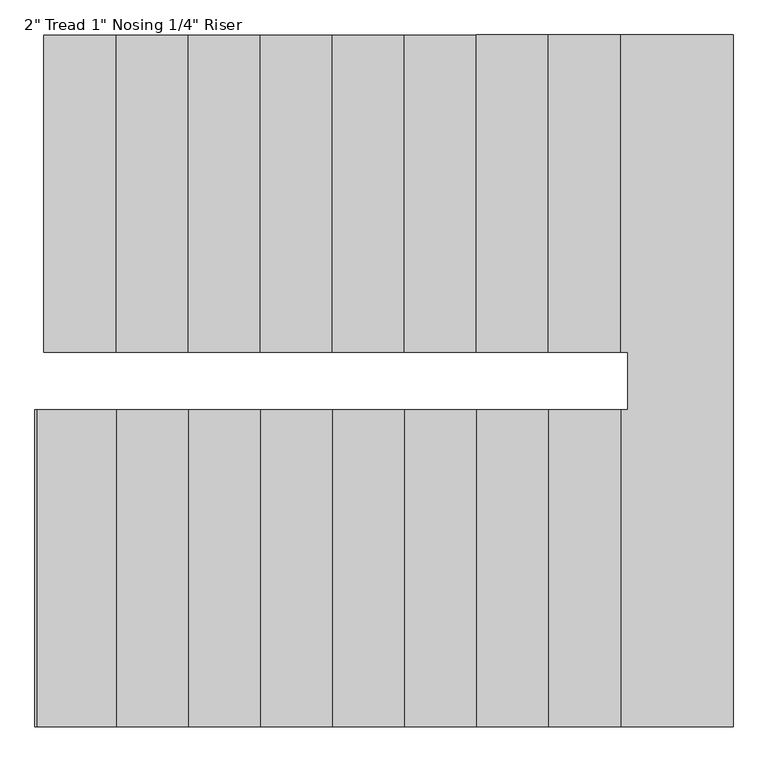
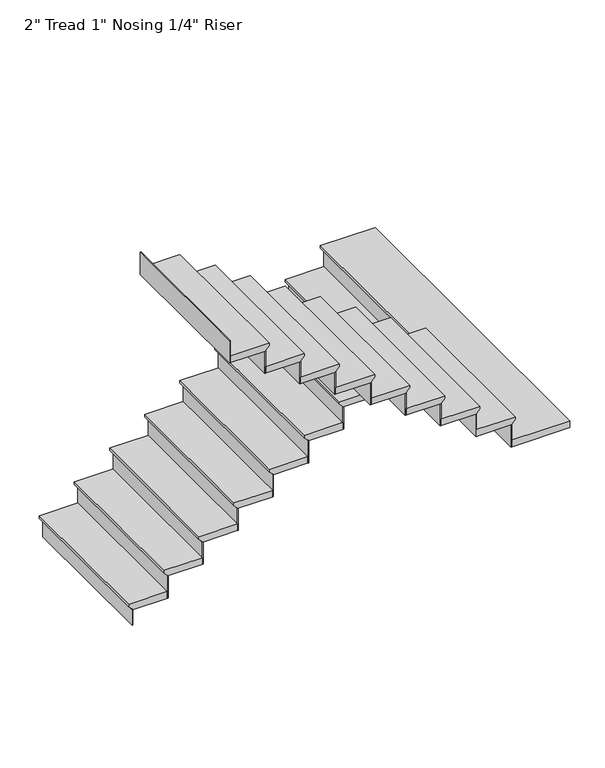
"""IFC4 building model written with IfcOpenShell, lengths in millimetres: stair flight geometry."""

from ifc_helpers import new_model, si_unit, origin, place, context, project, spatial, faceted_brep, source, transform, mapped, element, save


def stair_flight_b7e44e04(model_context):
    return source(origin(), model_context, "Body", "Brep", [
        faceted_brep([(-41148.2472477, 4654.7086027, 150.2833333), (-41148.2472477, 4654.7086027, 169.3333333), (-41148.2472477, 5772.3086027, 169.3333333), (-41148.2472477, 5772.3086027, 150.2833333), (-41122.8472477, 4654.7086027, 124.8833333), (-41122.8472477, 5772.3086027, 124.8833333), (-40868.8472477, 4654.7086027, 169.3333333), (-40868.8472477, 5772.3086027, 169.3333333), (-41122.8472477, 5772.3086027, 118.5333333), (-40868.8472477, 5772.3086027, 118.5333333), (-40868.8472477, 4654.7086027, 118.5333333), (-41122.8472477, 4654.7086027, 118.5333333)], [[[0, 1, 2, 3]], [[4, 0, 3, 5]], [[2, 1, 6, 7]], [[8, 9, 10, 11]], [[2, 7, 9, 8, 5, 3]], [[8, 11, 4, 5]], [[6, 1, 0, 4, 11, 10]], [[7, 6, 10, 9]]]),
        faceted_brep([(-41122.8472477, 4654.7086027, 118.5333333), (-41122.8472477, 4654.7086027, 0.0), (-41116.4972477, 4654.7086027, 0.0), (-41116.4972477, 4654.7086027, 118.5333333), (-41122.8472477, 5772.3086027, 118.5333333), (-41116.4972477, 5772.3086027, 118.5333333), (-41116.4972477, 5772.3086027, 0.0), (-41122.8472477, 5772.3086027, 0.0)], [[[0, 1, 2, 3]], [[4, 5, 6, 7]], [[1, 0, 4, 7]], [[2, 1, 7, 6]], [[3, 2, 6, 5]], [[0, 3, 5, 4]]]),
        faceted_brep([(-40868.8472477, 4654.7086027, 287.8666667), (-40868.8472477, 4654.7086027, 118.5333333), (-40862.4972477, 4654.7086027, 118.5333333), (-40862.4972477, 4654.7086027, 287.8666667), (-40868.8472477, 5772.3086027, 287.8666667), (-40862.4972477, 5772.3086027, 287.8666667), (-40862.4972477, 5772.3086027, 118.5333333), (-40868.8472477, 5772.3086027, 118.5333333)], [[[0, 1, 2, 3]], [[4, 5, 6, 7]], [[1, 0, 4, 7]], [[2, 1, 7, 6]], [[3, 2, 6, 5]], [[0, 3, 5, 4]]]),
        faceted_brep([(-40894.2472477, 5772.3086027, 338.6666667), (-40894.2472477, 4654.7086027, 338.6666667), (-40614.8472477, 4654.7086027, 338.6666667), (-40614.8472477, 5772.3086027, 338.6666667), (-40868.8472477, 5772.3086027, 287.8666667), (-40614.8472477, 5772.3086027, 287.8666667), (-40614.8472477, 4654.7086027, 287.8666667), (-40868.8472477, 4654.7086027, 287.8666667), (-40868.8472477, 5772.3086027, 294.2166667), (-40894.2472477, 5772.3086027, 319.6166667), (-40868.8472477, 4654.7086027, 294.2166667), (-40894.2472477, 4654.7086027, 319.6166667)], [[[0, 1, 2, 3]], [[4, 5, 6, 7]], [[0, 3, 5, 4, 8, 9]], [[4, 7, 10, 8]], [[2, 1, 11, 10, 7, 6]], [[3, 2, 6, 5]], [[11, 1, 0, 9]], [[10, 11, 9, 8]]]),
        faceted_brep([(-40614.8472477, 4654.7086027, 457.2), (-40614.8472477, 4654.7086027, 287.8666667), (-40608.4972477, 4654.7086027, 287.8666667), (-40608.4972477, 4654.7086027, 457.2), (-40614.8472477, 5772.3086027, 457.2), (-40608.4972477, 5772.3086027, 457.2), (-40608.4972477, 5772.3086027, 287.8666667), (-40614.8472477, 5772.3086027, 287.8666667)], [[[0, 1, 2, 3]], [[4, 5, 6, 7]], [[1, 0, 4, 7]], [[2, 1, 7, 6]], [[3, 2, 6, 5]], [[0, 3, 5, 4]]]),
        faceted_brep([(-40640.2472477, 5772.3086027, 508.0), (-40640.2472477, 4654.7086027, 508.0), (-40360.8472477, 4654.7086027, 508.0), (-40360.8472477, 5772.3086027, 508.0), (-40614.8472477, 5772.3086027, 457.2), (-40360.8472477, 5772.3086027, 457.2), (-40360.8472477, 4654.7086027, 457.2), (-40614.8472477, 4654.7086027, 457.2), (-40614.8472477, 5772.3086027, 463.55), (-40640.2472477, 5772.3086027, 488.95), (-40614.8472477, 4654.7086027, 463.55), (-40640.2472477, 4654.7086027, 488.95)], [[[0, 1, 2, 3]], [[4, 5, 6, 7]], [[0, 3, 5, 4, 8, 9]], [[4, 7, 10, 8]], [[2, 1, 11, 10, 7, 6]], [[3, 2, 6, 5]], [[11, 1, 0, 9]], [[10, 11, 9, 8]]]),
        faceted_brep([(-40360.8472477, 4654.7086027, 626.5333333), (-40360.8472477, 4654.7086027, 457.2), (-40354.4972477, 4654.7086027, 457.2), (-40354.4972477, 4654.7086027, 626.5333333), (-40360.8472477, 5772.3086027, 626.5333333), (-40354.4972477, 5772.3086027, 626.5333333), (-40354.4972477, 5772.3086027, 457.2), (-40360.8472477, 5772.3086027, 457.2)], [[[0, 1, 2, 3]], [[4, 5, 6, 7]], [[1, 0, 4, 7]], [[2, 1, 7, 6]], [[3, 2, 6, 5]], [[0, 3, 5, 4]]]),
        faceted_brep([(-40386.2472477, 5772.3086027, 677.3333333), (-40386.2472477, 4654.7086027, 677.3333333), (-40106.8472477, 4654.7086027, 677.3333333), (-40106.8472477, 5772.3086027, 677.3333333), (-40360.8472477, 5772.3086027, 626.5333333), (-40106.8472477, 5772.3086027, 626.5333333), (-40106.8472477, 4654.7086027, 626.5333333), (-40360.8472477, 4654.7086027, 626.5333333), (-40360.8472477, 5772.3086027, 632.8833333), (-40386.2472477, 5772.3086027, 658.2833333), (-40360.8472477, 4654.7086027, 632.8833333), (-40386.2472477, 4654.7086027, 658.2833333)], [[[0, 1, 2, 3]], [[4, 5, 6, 7]], [[0, 3, 5, 4, 8, 9]], [[4, 7, 10, 8]], [[2, 1, 11, 10, 7, 6]], [[3, 2, 6, 5]], [[11, 1, 0, 9]], [[10, 11, 9, 8]]]),
        faceted_brep([(-40106.8472477, 4654.7086027, 795.8666667), (-40106.8472477, 4654.7086027, 626.5333333), (-40100.4972477, 4654.7086027, 626.5333333), (-40100.4972477, 4654.7086027, 795.8666667), (-40106.8472477, 5772.3086027, 795.8666667), (-40100.4972477, 5772.3086027, 795.8666667), (-40100.4972477, 5772.3086027, 626.5333333), (-40106.8472477, 5772.3086027, 626.5333333)], [[[0, 1, 2, 3]], [[4, 5, 6, 7]], [[1, 0, 4, 7]], [[2, 1, 7, 6]], [[3, 2, 6, 5]], [[0, 3, 5, 4]]]),
        faceted_brep([(-40132.2472477, 5772.3086027, 846.6666667), (-40132.2472477, 4654.7086027, 846.6666667), (-39852.8472477, 4654.7086027, 846.6666667), (-39852.8472477, 5772.3086027, 846.6666667), (-40106.8472477, 5772.3086027, 795.8666667), (-39852.8472477, 5772.3086027, 795.8666667), (-39852.8472477, 4654.7086027, 795.8666667), (-40106.8472477, 4654.7086027, 795.8666667), (-40106.8472477, 5772.3086027, 802.2166667), (-40132.2472477, 5772.3086027, 827.6166667), (-40106.8472477, 4654.7086027, 802.2166667), (-40132.2472477, 4654.7086027, 827.6166667)], [[[0, 1, 2, 3]], [[4, 5, 6, 7]], [[0, 3, 5, 4, 8, 9]], [[4, 7, 10, 8]], [[2, 1, 11, 10, 7, 6]], [[3, 2, 6, 5]], [[11, 1, 0, 9]], [[10, 11, 9, 8]]]),
        faceted_brep([(-39852.8472477, 4654.7086027, 965.2), (-39852.8472477, 4654.7086027, 795.8666667), (-39846.4972477, 4654.7086027, 795.8666667), (-39846.4972477, 4654.7086027, 965.2), (-39852.8472477, 5772.3086027, 965.2), (-39846.4972477, 5772.3086027, 965.2), (-39846.4972477, 5772.3086027, 795.8666667), (-39852.8472477, 5772.3086027, 795.8666667)], [[[0, 1, 2, 3]], [[4, 5, 6, 7]], [[1, 0, 4, 7]], [[2, 1, 7, 6]], [[3, 2, 6, 5]], [[0, 3, 5, 4]]]),
        faceted_brep([(-39878.2472477, 5772.3086027, 1016.0), (-39878.2472477, 4654.7086027, 1016.0), (-39598.8472477, 4654.7086027, 1016.0), (-39598.8472477, 5772.3086027, 1016.0), (-39852.8472477, 5772.3086027, 965.2), (-39598.8472477, 5772.3086027, 965.2), (-39598.8472477, 4654.7086027, 965.2), (-39852.8472477, 4654.7086027, 965.2), (-39852.8472477, 5772.3086027, 971.55), (-39878.2472477, 5772.3086027, 996.95), (-39852.8472477, 4654.7086027, 971.55), (-39878.2472477, 4654.7086027, 996.95)], [[[0, 1, 2, 3]], [[4, 5, 6, 7]], [[0, 3, 5, 4, 8, 9]], [[4, 7, 10, 8]], [[2, 1, 11, 10, 7, 6]], [[3, 2, 6, 5]], [[11, 1, 0, 9]], [[10, 11, 9, 8]]]),
        faceted_brep([(-39598.8472477, 4654.7086027, 1134.5333333), (-39598.8472477, 4654.7086027, 965.2), (-39592.4972477, 4654.7086027, 965.2), (-39592.4972477, 4654.7086027, 1134.5333333), (-39598.8472477, 5772.3086027, 1134.5333333), (-39592.4972477, 5772.3086027, 1134.5333333), (-39592.4972477, 5772.3086027, 965.2), (-39598.8472477, 5772.3086027, 965.2)], [[[0, 1, 2, 3]], [[4, 5, 6, 7]], [[1, 0, 4, 7]], [[2, 1, 7, 6]], [[3, 2, 6, 5]], [[0, 3, 5, 4]]]),
        faceted_brep([(-39624.2472477, 5772.3086027, 1185.3333333), (-39624.2472477, 4654.7086027, 1185.3333333), (-39344.8472477, 4654.7086027, 1185.3333333), (-39344.8472477, 5772.3086027, 1185.3333333), (-39598.8472477, 5772.3086027, 1134.5333333), (-39344.8472477, 5772.3086027, 1134.5333333), (-39344.8472477, 4654.7086027, 1134.5333333), (-39598.8472477, 4654.7086027, 1134.5333333), (-39598.8472477, 5772.3086027, 1140.8833333), (-39624.2472477, 5772.3086027, 1166.2833333), (-39598.8472477, 4654.7086027, 1140.8833333), (-39624.2472477, 4654.7086027, 1166.2833333)], [[[0, 1, 2, 3]], [[4, 5, 6, 7]], [[0, 3, 5, 4, 8, 9]], [[4, 7, 10, 8]], [[2, 1, 11, 10, 7, 6]], [[3, 2, 6, 5]], [[11, 1, 0, 9]], [[10, 11, 9, 8]]]),
        faceted_brep([(-39344.8472477, 4654.7086027, 1303.8666667), (-39344.8472477, 4654.7086027, 1134.5333333), (-39338.4972477, 4654.7086027, 1134.5333333), (-39338.4972477, 4654.7086027, 1303.8666667), (-39344.8472477, 5772.3086027, 1303.8666667), (-39338.4972477, 5772.3086027, 1303.8666667), (-39338.4972477, 5772.3086027, 1134.5333333), (-39344.8472477, 5772.3086027, 1134.5333333)], [[[0, 1, 2, 3]], [[4, 5, 6, 7]], [[1, 0, 4, 7]], [[2, 1, 7, 6]], [[3, 2, 6, 5]], [[0, 3, 5, 4]]]),
        faceted_brep([(-39370.2472477, 5772.3086027, 1354.6666667), (-39370.2472477, 4654.7086027, 1354.6666667), (-39090.8472477, 4654.7086027, 1354.6666667), (-39090.8472477, 5772.3086027, 1354.6666667), (-39344.8472477, 5772.3086027, 1303.8666667), (-39090.8472477, 5772.3086027, 1303.8666667), (-39090.8472477, 4654.7086027, 1303.8666667), (-39344.8472477, 4654.7086027, 1303.8666667), (-39344.8472477, 5772.3086027, 1310.2166667), (-39370.2472477, 5772.3086027, 1335.6166667), (-39344.8472477, 4654.7086027, 1310.2166667), (-39370.2472477, 4654.7086027, 1335.6166667)], [[[0, 1, 2, 3]], [[4, 5, 6, 7]], [[0, 3, 5, 4, 8, 9]], [[4, 7, 10, 8]], [[2, 1, 11, 10, 7, 6]], [[3, 2, 6, 5]], [[11, 1, 0, 9]], [[10, 11, 9, 8]]]),
        faceted_brep([(-39090.8472477, 4654.7086027, 1473.2), (-39090.8472477, 4654.7086027, 1303.8666667), (-39084.4972477, 4654.7086027, 1303.8666667), (-39084.4972477, 4654.7086027, 1473.2), (-39090.8472477, 5772.3086027, 1473.2), (-39084.4972477, 5772.3086027, 1473.2), (-39084.4972477, 5772.3086027, 1303.8666667), (-39090.8472477, 5772.3086027, 1303.8666667)], [[[0, 1, 2, 3]], [[4, 5, 6, 7]], [[1, 0, 4, 7]], [[2, 1, 7, 6]], [[3, 2, 6, 5]], [[0, 3, 5, 4]]]),
        faceted_brep([(-39141.6472477, 3333.9086027, 1524.0), (-38719.7380314, 3333.9086027, 1524.0), (-38719.7380314, 5772.3086027, 1524.0), (-39116.2472477, 5772.3086027, 1524.0), (-39116.2472477, 4654.7086027, 1524.0), (-39090.8472477, 4654.7086027, 1524.0), (-39090.8472477, 4451.5086027, 1524.0), (-39141.6472477, 4451.5086027, 1524.0), (-38719.7380314, 3333.9086027, 1473.2), (-39141.6472477, 3333.9086027, 1473.2), (-39141.6472477, 4451.5086027, 1473.2), (-39090.8472477, 4451.5086027, 1473.2), (-39090.8472477, 4654.7086027, 1473.2), (-39090.8472477, 5772.3086027, 1473.2), (-38719.7380314, 5772.3086027, 1473.2), (-39090.8472477, 5772.3086027, 1479.55), (-39116.2472477, 5772.3086027, 1504.95), (-39090.8472477, 4654.7086027, 1479.55), (-39116.2472477, 4654.7086027, 1504.95)], [[[0, 1, 2, 3, 4, 5, 6, 7]], [[8, 9, 10, 11, 12, 13, 14]], [[1, 0, 9, 8]], [[2, 1, 8, 14]], [[3, 2, 14, 13, 15, 16]], [[13, 12, 17, 15]], [[6, 5, 17, 12, 11]], [[7, 6, 11, 10]], [[0, 7, 10, 9]], [[4, 18, 17, 5]], [[18, 4, 3, 16]], [[17, 18, 16, 15]]]),
        faceted_brep([(-39141.6472477, 4451.5086027, 1642.5333333), (-39141.6472477, 4451.5086027, 1473.2), (-39147.9972477, 4451.5086027, 1473.2), (-39147.9972477, 4451.5086027, 1642.5333333), (-39141.6472477, 3333.9086027, 1642.5333333), (-39147.9972477, 3333.9086027, 1642.5333333), (-39147.9972477, 3333.9086027, 1473.2), (-39141.6472477, 3333.9086027, 1473.2)], [[[0, 1, 2, 3]], [[4, 5, 6, 7]], [[1, 0, 4, 7]], [[2, 1, 7, 6]], [[3, 2, 6, 5]], [[0, 3, 5, 4]]]),
        faceted_brep([(-39116.2472477, 3333.9086027, 1693.3333333), (-39116.2472477, 4451.5086027, 1693.3333333), (-39395.6472477, 4451.5086027, 1693.3333333), (-39395.6472477, 3333.9086027, 1693.3333333), (-39141.6472477, 3333.9086027, 1642.5333333), (-39395.6472477, 3333.9086027, 1642.5333333), (-39395.6472477, 4451.5086027, 1642.5333333), (-39141.6472477, 4451.5086027, 1642.5333333), (-39141.6472477, 3333.9086027, 1648.8833333), (-39116.2472477, 3333.9086027, 1674.2833333), (-39141.6472477, 4451.5086027, 1648.8833333), (-39116.2472477, 4451.5086027, 1674.2833333)], [[[0, 1, 2, 3]], [[4, 5, 6, 7]], [[0, 3, 5, 4, 8, 9]], [[4, 7, 10, 8]], [[2, 1, 11, 10, 7, 6]], [[3, 2, 6, 5]], [[11, 1, 0, 9]], [[10, 11, 9, 8]]]),
        faceted_brep([(-39395.6472477, 4451.5086027, 1811.8666667), (-39395.6472477, 4451.5086027, 1642.5333333), (-39401.9972477, 4451.5086027, 1642.5333333), (-39401.9972477, 4451.5086027, 1811.8666667), (-39395.6472477, 3333.9086027, 1811.8666667), (-39401.9972477, 3333.9086027, 1811.8666667), (-39401.9972477, 3333.9086027, 1642.5333333), (-39395.6472477, 3333.9086027, 1642.5333333)], [[[0, 1, 2, 3]], [[4, 5, 6, 7]], [[1, 0, 4, 7]], [[2, 1, 7, 6]], [[3, 2, 6, 5]], [[0, 3, 5, 4]]]),
        faceted_brep([(-39370.2472477, 3333.9086027, 1862.6666667), (-39370.2472477, 4451.5086027, 1862.6666667), (-39649.6472477, 4451.5086027, 1862.6666667), (-39649.6472477, 3333.9086027, 1862.6666667), (-39395.6472477, 3333.9086027, 1811.8666667), (-39649.6472477, 3333.9086027, 1811.8666667), (-39649.6472477, 4451.5086027, 1811.8666667), (-39395.6472477, 4451.5086027, 1811.8666667), (-39395.6472477, 3333.9086027, 1818.2166667), (-39370.2472477, 3333.9086027, 1843.6166667), (-39395.6472477, 4451.5086027, 1818.2166667), (-39370.2472477, 4451.5086027, 1843.6166667)], [[[0, 1, 2, 3]], [[4, 5, 6, 7]], [[0, 3, 5, 4, 8, 9]], [[4, 7, 10, 8]], [[2, 1, 11, 10, 7, 6]], [[3, 2, 6, 5]], [[11, 1, 0, 9]], [[10, 11, 9, 8]]]),
        faceted_brep([(-39649.6472477, 4451.5086027, 1981.2), (-39649.6472477, 4451.5086027, 1811.8666667), (-39655.9972477, 4451.5086027, 1811.8666667), (-39655.9972477, 4451.5086027, 1981.2), (-39649.6472477, 3333.9086027, 1981.2), (-39655.9972477, 3333.9086027, 1981.2), (-39655.9972477, 3333.9086027, 1811.8666667), (-39649.6472477, 3333.9086027, 1811.8666667)], [[[0, 1, 2, 3]], [[4, 5, 6, 7]], [[1, 0, 4, 7]], [[2, 1, 7, 6]], [[3, 2, 6, 5]], [[0, 3, 5, 4]]]),
        faceted_brep([(-39624.2472477, 3333.9086027, 2032.0), (-39624.2472477, 4451.5086027, 2032.0), (-39903.6472477, 4451.5086027, 2032.0), (-39903.6472477, 3333.9086027, 2032.0), (-39649.6472477, 3333.9086027, 1981.2), (-39903.6472477, 3333.9086027, 1981.2), (-39903.6472477, 4451.5086027, 1981.2), (-39649.6472477, 4451.5086027, 1981.2), (-39649.6472477, 3333.9086027, 1987.55), (-39624.2472477, 3333.9086027, 2012.95), (-39649.6472477, 4451.5086027, 1987.55), (-39624.2472477, 4451.5086027, 2012.95)], [[[0, 1, 2, 3]], [[4, 5, 6, 7]], [[0, 3, 5, 4, 8, 9]], [[4, 7, 10, 8]], [[2, 1, 11, 10, 7, 6]], [[3, 2, 6, 5]], [[11, 1, 0, 9]], [[10, 11, 9, 8]]]),
        faceted_brep([(-39903.6472477, 4451.5086027, 2150.5333333), (-39903.6472477, 4451.5086027, 1981.2), (-39909.9972477, 4451.5086027, 1981.2), (-39909.9972477, 4451.5086027, 2150.5333333), (-39903.6472477, 3333.9086027, 2150.5333333), (-39909.9972477, 3333.9086027, 2150.5333333), (-39909.9972477, 3333.9086027, 1981.2), (-39903.6472477, 3333.9086027, 1981.2)], [[[0, 1, 2, 3]], [[4, 5, 6, 7]], [[1, 0, 4, 7]], [[2, 1, 7, 6]], [[3, 2, 6, 5]], [[0, 3, 5, 4]]]),
        faceted_brep([(-39878.2472477, 3333.9086027, 2201.3333333), (-39878.2472477, 4451.5086027, 2201.3333333), (-40157.6472477, 4451.5086027, 2201.3333333), (-40157.6472477, 3333.9086027, 2201.3333333), (-39903.6472477, 3333.9086027, 2150.5333333), (-40157.6472477, 3333.9086027, 2150.5333333), (-40157.6472477, 4451.5086027, 2150.5333333), (-39903.6472477, 4451.5086027, 2150.5333333), (-39903.6472477, 3333.9086027, 2156.8833333), (-39878.2472477, 3333.9086027, 2182.2833333), (-39903.6472477, 4451.5086027, 2156.8833333), (-39878.2472477, 4451.5086027, 2182.2833333)], [[[0, 1, 2, 3]], [[4, 5, 6, 7]], [[0, 3, 5, 4, 8, 9]], [[4, 7, 10, 8]], [[2, 1, 11, 10, 7, 6]], [[3, 2, 6, 5]], [[11, 1, 0, 9]], [[10, 11, 9, 8]]]),
        faceted_brep([(-40157.6472477, 4451.5086027, 2319.8666667), (-40157.6472477, 4451.5086027, 2150.5333333), (-40163.9972477, 4451.5086027, 2150.5333333), (-40163.9972477, 4451.5086027, 2319.8666667), (-40157.6472477, 3333.9086027, 2319.8666667), (-40163.9972477, 3333.9086027, 2319.8666667), (-40163.9972477, 3333.9086027, 2150.5333333), (-40157.6472477, 3333.9086027, 2150.5333333)], [[[0, 1, 2, 3]], [[4, 5, 6, 7]], [[1, 0, 4, 7]], [[2, 1, 7, 6]], [[3, 2, 6, 5]], [[0, 3, 5, 4]]]),
        faceted_brep([(-40132.2472477, 3333.9086027, 2370.6666667), (-40132.2472477, 4451.5086027, 2370.6666667), (-40411.6472477, 4451.5086027, 2370.6666667), (-40411.6472477, 3333.9086027, 2370.6666667), (-40157.6472477, 3333.9086027, 2319.8666667), (-40411.6472477, 3333.9086027, 2319.8666667), (-40411.6472477, 4451.5086027, 2319.8666667), (-40157.6472477, 4451.5086027, 2319.8666667), (-40157.6472477, 3333.9086027, 2326.2166667), (-40132.2472477, 3333.9086027, 2351.6166667), (-40157.6472477, 4451.5086027, 2326.2166667), (-40132.2472477, 4451.5086027, 2351.6166667)], [[[0, 1, 2, 3]], [[4, 5, 6, 7]], [[0, 3, 5, 4, 8, 9]], [[4, 7, 10, 8]], [[2, 1, 11, 10, 7, 6]], [[3, 2, 6, 5]], [[11, 1, 0, 9]], [[10, 11, 9, 8]]]),
        faceted_brep([(-40411.6472477, 4451.5086027, 2489.2), (-40411.6472477, 4451.5086027, 2319.8666667), (-40417.9972477, 4451.5086027, 2319.8666667), (-40417.9972477, 4451.5086027, 2489.2), (-40411.6472477, 3333.9086027, 2489.2), (-40417.9972477, 3333.9086027, 2489.2), (-40417.9972477, 3333.9086027, 2319.8666667), (-40411.6472477, 3333.9086027, 2319.8666667)], [[[0, 1, 2, 3]], [[4, 5, 6, 7]], [[1, 0, 4, 7]], [[2, 1, 7, 6]], [[3, 2, 6, 5]], [[0, 3, 5, 4]]]),
        faceted_brep([(-40386.2472477, 3333.9086027, 2540.0), (-40386.2472477, 4451.5086027, 2540.0), (-40665.6472477, 4451.5086027, 2540.0), (-40665.6472477, 3333.9086027, 2540.0), (-40411.6472477, 3333.9086027, 2489.2), (-40665.6472477, 3333.9086027, 2489.2), (-40665.6472477, 4451.5086027, 2489.2), (-40411.6472477, 4451.5086027, 2489.2), (-40411.6472477, 3333.9086027, 2495.55), (-40386.2472477, 3333.9086027, 2520.95), (-40411.6472477, 4451.5086027, 2495.55), (-40386.2472477, 4451.5086027, 2520.95)], [[[0, 1, 2, 3]], [[4, 5, 6, 7]], [[0, 3, 5, 4, 8, 9]], [[4, 7, 10, 8]], [[2, 1, 11, 10, 7, 6]], [[3, 2, 6, 5]], [[11, 1, 0, 9]], [[10, 11, 9, 8]]]),
        faceted_brep([(-40665.6472477, 4451.5086027, 2658.5333333), (-40665.6472477, 4451.5086027, 2489.2), (-40671.9972477, 4451.5086027, 2489.2), (-40671.9972477, 4451.5086027, 2658.5333333), (-40665.6472477, 3333.9086027, 2658.5333333), (-40671.9972477, 3333.9086027, 2658.5333333), (-40671.9972477, 3333.9086027, 2489.2), (-40665.6472477, 3333.9086027, 2489.2)], [[[0, 1, 2, 3]], [[4, 5, 6, 7]], [[1, 0, 4, 7]], [[2, 1, 7, 6]], [[3, 2, 6, 5]], [[0, 3, 5, 4]]]),
        faceted_brep([(-40640.2472477, 3333.9086027, 2709.3333333), (-40640.2472477, 4451.5086027, 2709.3333333), (-40919.6472477, 4451.5086027, 2709.3333333), (-40919.6472477, 3333.9086027, 2709.3333333), (-40665.6472477, 3333.9086027, 2658.5333333), (-40919.6472477, 3333.9086027, 2658.5333333), (-40919.6472477, 4451.5086027, 2658.5333333), (-40665.6472477, 4451.5086027, 2658.5333333), (-40665.6472477, 3333.9086027, 2664.8833333), (-40640.2472477, 3333.9086027, 2690.2833333), (-40665.6472477, 4451.5086027, 2664.8833333), (-40640.2472477, 4451.5086027, 2690.2833333)], [[[0, 1, 2, 3]], [[4, 5, 6, 7]], [[0, 3, 5, 4, 8, 9]], [[4, 7, 10, 8]], [[2, 1, 11, 10, 7, 6]], [[3, 2, 6, 5]], [[11, 1, 0, 9]], [[10, 11, 9, 8]]]),
        faceted_brep([(-40919.6472477, 4451.5086027, 2827.8666667), (-40919.6472477, 4451.5086027, 2658.5333333), (-40925.9972477, 4451.5086027, 2658.5333333), (-40925.9972477, 4451.5086027, 2827.8666667), (-40919.6472477, 3333.9086027, 2827.8666667), (-40925.9972477, 3333.9086027, 2827.8666667), (-40925.9972477, 3333.9086027, 2658.5333333), (-40919.6472477, 3333.9086027, 2658.5333333)], [[[0, 1, 2, 3]], [[4, 5, 6, 7]], [[1, 0, 4, 7]], [[2, 1, 7, 6]], [[3, 2, 6, 5]], [[0, 3, 5, 4]]]),
        faceted_brep([(-41173.6472477, 4451.5086027, 2997.2), (-41173.6472477, 4451.5086027, 2827.8666667), (-41179.9972477, 4451.5086027, 2827.8666667), (-41179.9972477, 4451.5086027, 2997.2), (-41173.6472477, 3333.9086027, 2997.2), (-41179.9972477, 3333.9086027, 2997.2), (-41179.9972477, 3333.9086027, 2827.8666667), (-41173.6472477, 3333.9086027, 2827.8666667)], [[[0, 1, 2, 3]], [[4, 5, 6, 7]], [[1, 0, 4, 7]], [[2, 1, 7, 6]], [[3, 2, 6, 5]], [[0, 3, 5, 4]]]),
        faceted_brep([(-40894.2472477, 3333.9086027, 2878.6666667), (-40894.2472477, 4451.5086027, 2878.6666667), (-41173.6472477, 4451.5086027, 2878.6666667), (-41173.6472477, 3333.9086027, 2878.6666667), (-40919.6472477, 3333.9086027, 2827.8666667), (-41173.6472477, 3333.9086027, 2827.8666667), (-41173.6472477, 4451.5086027, 2827.8666667), (-40919.6472477, 4451.5086027, 2827.8666667), (-40919.6472477, 3333.9086027, 2834.2166667), (-40894.2472477, 3333.9086027, 2859.6166667), (-40919.6472477, 4451.5086027, 2834.2166667), (-40894.2472477, 4451.5086027, 2859.6166667)], [[[0, 1, 2, 3]], [[4, 5, 6, 7]], [[0, 3, 5, 4, 8, 9]], [[4, 7, 10, 8]], [[2, 1, 11, 10, 7, 6]], [[3, 2, 6, 5]], [[11, 1, 0, 9]], [[10, 11, 9, 8]]]),
    ])


if __name__ == "__main__":
    model = new_model("IFC4")
    model_context = context("Model", 3, world=origin())
    ifc_project = project(units=[si_unit("LENGTHUNIT", "METRE", prefix="MILLI")], contexts=[model_context])
    site = spatial("IfcSite", under=ifc_project)
    building = spatial("IfcBuilding", under=site)
    placement = place(None, origin())
    stair_flight_shape = stair_flight_b7e44e04(model_context)
    element("IfcStairFlight", 1, ObjectType="2\" Tread 1\" Nosing 1/4\" Riser", at=placement, inside=building, context=model_context, shape_type="MappedRepresentation", body=[
        mapped(stair_flight_shape, transform((0.0, 0.0, 0.0), x_axis=(1.0, 0.0, 0.0), y_axis=(0.0, 1.0, 0.0), z_axis=(0.0, 0.0, 1.0))),
    ])
    save(model, "model.ifc")
